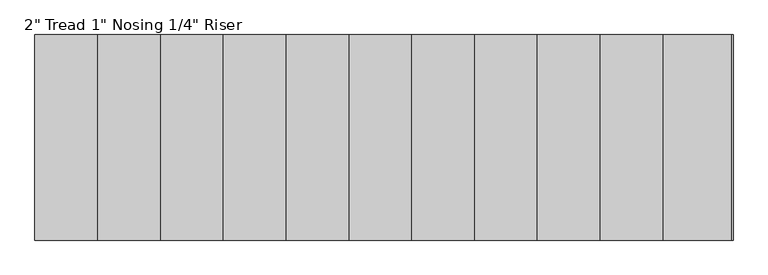
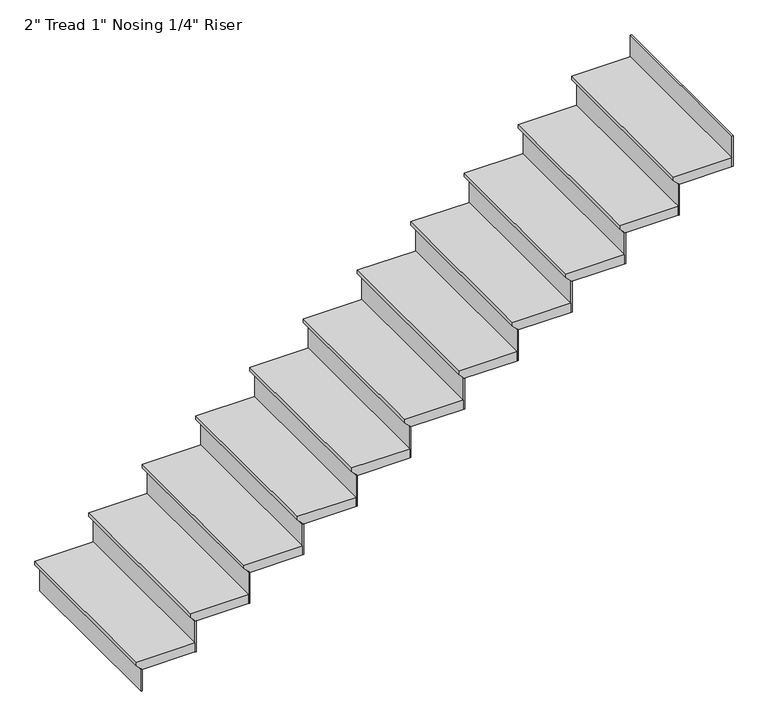
"""IFC4 building model written with IfcOpenShell, lengths in millimetres: stair flight geometry."""

from ifc_helpers import new_model, si_unit, frame, origin, origin_with_axes, place, context, project, spatial, polyline, outline, extrude, source, transform, mapped, element, save


def stair_flight_ef017676(model_context):
    return source(origin(), model_context, "Body", "SweptSolid", [
        extrude(outline(polyline([(169.3333333, -4095.9663486), (169.3333333, -4400.7663486), (150.2833333, -4400.7663486), (124.8833333, -4375.3663486), (118.5333333, -4375.3663486), (118.5333333, -4095.9663486), (169.3333333, -4095.9663486)])), frame((0.0, 1993.3117215, 0.0), z_axis=(0.0, 1.0, 0.0), x_axis=(0.0, 0.0, 1.0)), (0.0, 0.0, 1.0), 914.4),
        extrude(outline(polyline([(-4369.0163486, 1993.3117215), (-4375.3663486, 1993.3117215), (-4375.3663486, 2907.7117215), (-4369.0163486, 2907.7117215), (-4369.0163486, 1993.3117215)])), origin_with_axes(), (0.0, 0.0, 1.0), 118.5333333),
        extrude(outline(polyline([(-4089.6163486, 1993.3117215), (-4095.9663486, 1993.3117215), (-4095.9663486, 2907.7117215), (-4089.6163486, 2907.7117215), (-4089.6163486, 1993.3117215)])), frame((0.0, 0.0, 118.5333333), z_axis=(0.0, 0.0, 1.0), x_axis=(1.0, 0.0, 0.0)), (0.0, 0.0, 1.0), 169.3333333),
        extrude(outline(polyline([(338.6666667, -3816.5663486), (338.6666667, -4121.3663486), (319.6166667, -4121.3663486), (294.2166667, -4095.9663486), (287.8666667, -4095.9663486), (287.8666667, -3816.5663486), (338.6666667, -3816.5663486)])), frame((0.0, 1993.3117215, 0.0), z_axis=(0.0, 1.0, 0.0), x_axis=(0.0, 0.0, 1.0)), (0.0, 0.0, 1.0), 914.4),
        extrude(outline(polyline([(-3810.2163486, 1993.3117215), (-3816.5663486, 1993.3117215), (-3816.5663486, 2907.7117215), (-3810.2163486, 2907.7117215), (-3810.2163486, 1993.3117215)])), frame((0.0, 0.0, 287.8666667), z_axis=(0.0, 0.0, 1.0), x_axis=(1.0, 0.0, 0.0)), (0.0, 0.0, 1.0), 169.3333333),
        extrude(outline(polyline([(508.0, -3537.1663486), (508.0, -3841.9663486), (488.95, -3841.9663486), (463.55, -3816.5663486), (457.2, -3816.5663486), (457.2, -3537.1663486), (508.0, -3537.1663486)])), frame((0.0, 1993.3117215, 0.0), z_axis=(0.0, 1.0, 0.0), x_axis=(0.0, 0.0, 1.0)), (0.0, 0.0, 1.0), 914.4),
        extrude(outline(polyline([(-3530.8163486, 1993.3117215), (-3537.1663486, 1993.3117215), (-3537.1663486, 2907.7117215), (-3530.8163486, 2907.7117215), (-3530.8163486, 1993.3117215)])), frame((0.0, 0.0, 457.2), z_axis=(0.0, 0.0, 1.0), x_axis=(1.0, 0.0, 0.0)), (0.0, 0.0, 1.0), 169.3333333),
        extrude(outline(polyline([(677.3333333, -3257.7663486), (677.3333333, -3562.5663486), (658.2833333, -3562.5663486), (632.8833333, -3537.1663486), (626.5333333, -3537.1663486), (626.5333333, -3257.7663486), (677.3333333, -3257.7663486)])), frame((0.0, 1993.3117215, 0.0), z_axis=(0.0, 1.0, 0.0), x_axis=(0.0, 0.0, 1.0)), (0.0, 0.0, 1.0), 914.4),
        extrude(outline(polyline([(-3251.4163486, 1993.3117215), (-3257.7663486, 1993.3117215), (-3257.7663486, 2907.7117215), (-3251.4163486, 2907.7117215), (-3251.4163486, 1993.3117215)])), frame((0.0, 0.0, 626.5333333), z_axis=(0.0, 0.0, 1.0), x_axis=(1.0, 0.0, 0.0)), (0.0, 0.0, 1.0), 169.3333333),
        extrude(outline(polyline([(846.6666667, -2978.3663486), (846.6666667, -3283.1663486), (827.6166667, -3283.1663486), (802.2166667, -3257.7663486), (795.8666667, -3257.7663486), (795.8666667, -2978.3663486), (846.6666667, -2978.3663486)])), frame((0.0, 1993.3117215, 0.0), z_axis=(0.0, 1.0, 0.0), x_axis=(0.0, 0.0, 1.0)), (0.0, 0.0, 1.0), 914.4),
        extrude(outline(polyline([(-2972.0163486, 1993.3117215), (-2978.3663486, 1993.3117215), (-2978.3663486, 2907.7117215), (-2972.0163486, 2907.7117215), (-2972.0163486, 1993.3117215)])), frame((0.0, 0.0, 795.8666667), z_axis=(0.0, 0.0, 1.0), x_axis=(1.0, 0.0, 0.0)), (0.0, 0.0, 1.0), 169.3333333),
        extrude(outline(polyline([(1016.0, -2698.9663486), (1016.0, -3003.7663486), (996.95, -3003.7663486), (971.55, -2978.3663486), (965.2, -2978.3663486), (965.2, -2698.9663486), (1016.0, -2698.9663486)])), frame((0.0, 1993.3117215, 0.0), z_axis=(0.0, 1.0, 0.0), x_axis=(0.0, 0.0, 1.0)), (0.0, 0.0, 1.0), 914.4),
        extrude(outline(polyline([(-2692.6163486, 1993.3117215), (-2698.9663486, 1993.3117215), (-2698.9663486, 2907.7117215), (-2692.6163486, 2907.7117215), (-2692.6163486, 1993.3117215)])), frame((0.0, 0.0, 965.2), z_axis=(0.0, 0.0, 1.0), x_axis=(1.0, 0.0, 0.0)), (0.0, 0.0, 1.0), 169.3333333),
        extrude(outline(polyline([(1185.3333333, -2419.5663486), (1185.3333333, -2724.3663486), (1166.2833333, -2724.3663486), (1140.8833333, -2698.9663486), (1134.5333333, -2698.9663486), (1134.5333333, -2419.5663486), (1185.3333333, -2419.5663486)])), frame((0.0, 1993.3117215, 0.0), z_axis=(0.0, 1.0, 0.0), x_axis=(0.0, 0.0, 1.0)), (0.0, 0.0, 1.0), 914.4),
        extrude(outline(polyline([(-2413.2163486, 1993.3117215), (-2419.5663486, 1993.3117215), (-2419.5663486, 2907.7117215), (-2413.2163486, 2907.7117215), (-2413.2163486, 1993.3117215)])), frame((0.0, 0.0, 1134.5333333), z_axis=(0.0, 0.0, 1.0), x_axis=(1.0, 0.0, 0.0)), (0.0, 0.0, 1.0), 169.3333333),
        extrude(outline(polyline([(1354.6666667, -2140.1663486), (1354.6666667, -2444.9663486), (1335.6166667, -2444.9663486), (1310.2166667, -2419.5663486), (1303.8666667, -2419.5663486), (1303.8666667, -2140.1663486), (1354.6666667, -2140.1663486)])), frame((0.0, 1993.3117215, 0.0), z_axis=(0.0, 1.0, 0.0), x_axis=(0.0, 0.0, 1.0)), (0.0, 0.0, 1.0), 914.4),
        extrude(outline(polyline([(-2133.8163486, 1993.3117215), (-2140.1663486, 1993.3117215), (-2140.1663486, 2907.7117215), (-2133.8163486, 2907.7117215), (-2133.8163486, 1993.3117215)])), frame((0.0, 0.0, 1303.8666667), z_axis=(0.0, 0.0, 1.0), x_axis=(1.0, 0.0, 0.0)), (0.0, 0.0, 1.0), 169.3333333),
        extrude(outline(polyline([(1524.0, -1860.7663486), (1524.0, -2165.5663486), (1504.95, -2165.5663486), (1479.55, -2140.1663486), (1473.2, -2140.1663486), (1473.2, -1860.7663486), (1524.0, -1860.7663486)])), frame((0.0, 1993.3117215, 0.0), z_axis=(0.0, 1.0, 0.0), x_axis=(0.0, 0.0, 1.0)), (0.0, 0.0, 1.0), 914.4),
        extrude(outline(polyline([(-1854.4163486, 1993.3117215), (-1860.7663486, 1993.3117215), (-1860.7663486, 2907.7117215), (-1854.4163486, 2907.7117215), (-1854.4163486, 1993.3117215)])), frame((0.0, 0.0, 1473.2), z_axis=(0.0, 0.0, 1.0), x_axis=(1.0, 0.0, 0.0)), (0.0, 0.0, 1.0), 169.3333333),
        extrude(outline(polyline([(1693.3333333, -1581.3663486), (1693.3333333, -1886.1663486), (1674.2833333, -1886.1663486), (1648.8833333, -1860.7663486), (1642.5333333, -1860.7663486), (1642.5333333, -1581.3663486), (1693.3333333, -1581.3663486)])), frame((0.0, 1993.3117215, 0.0), z_axis=(0.0, 1.0, 0.0), x_axis=(0.0, 0.0, 1.0)), (0.0, 0.0, 1.0), 914.4),
        extrude(outline(polyline([(-1575.0163486, 1993.3117215), (-1581.3663486, 1993.3117215), (-1581.3663486, 2907.7117215), (-1575.0163486, 2907.7117215), (-1575.0163486, 1993.3117215)])), frame((0.0, 0.0, 1642.5333333), z_axis=(0.0, 0.0, 1.0), x_axis=(1.0, 0.0, 0.0)), (0.0, 0.0, 1.0), 169.3333333),
        extrude(outline(polyline([(-1295.6163486, 1993.3117215), (-1301.9663486, 1993.3117215), (-1301.9663486, 2907.7117215), (-1295.6163486, 2907.7117215), (-1295.6163486, 1993.3117215)])), frame((0.0, 0.0, 1811.8666667), z_axis=(0.0, 0.0, 1.0), x_axis=(1.0, 0.0, 0.0)), (0.0, 0.0, 1.0), 169.3333333),
        extrude(outline(polyline([(1862.6666667, -1301.9663486), (1862.6666667, -1606.7663486), (1843.6166667, -1606.7663486), (1818.2166667, -1581.3663486), (1811.8666667, -1581.3663486), (1811.8666667, -1301.9663486), (1862.6666667, -1301.9663486)])), frame((0.0, 1993.3117215, 0.0), z_axis=(0.0, 1.0, 0.0), x_axis=(0.0, 0.0, 1.0)), (0.0, 0.0, 1.0), 914.4),
    ])


if __name__ == "__main__":
    model = new_model("IFC4")
    model_context = context("Model", 3, world=origin())
    ifc_project = project(units=[si_unit("LENGTHUNIT", "METRE", prefix="MILLI")], contexts=[model_context])
    site = spatial("IfcSite", under=ifc_project)
    building = spatial("IfcBuilding", under=site)
    placement = place(None, origin())
    stair_flight_shape = stair_flight_ef017676(model_context)
    element("IfcStairFlight", 1, ObjectType="2\" Tread 1\" Nosing 1/4\" Riser", at=placement, inside=building, context=model_context, shape_type="MappedRepresentation", body=[
        mapped(stair_flight_shape, transform((0.0, 0.0, 0.0), x_axis=(1.0, 0.0, 0.0), y_axis=(0.0, 1.0, 0.0), z_axis=(0.0, 0.0, 1.0))),
    ])
    save(model, "model.ifc")
